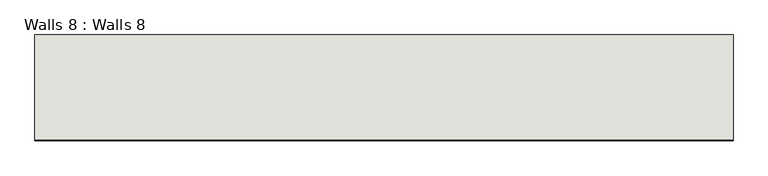
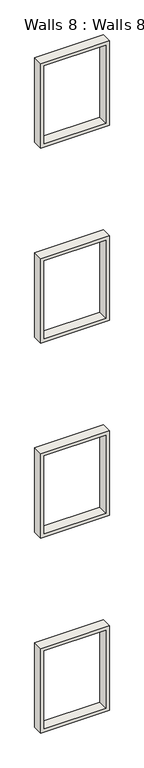
"""IFC4 building model written with IfcOpenShell, lengths in millimetres: wall geometry, Walls 8 : Walls 8."""

from ifc_helpers import new_model, si_unit, frame, origin, place, context, project, spatial, polyline, outline, extrude, source, transform, mapped, element, save


def walls_8_walls_8_31a24d2c(model_context):
    return source(origin(), model_context, "Body", "SweptSolid", [
        extrude(outline(polyline([(13030.2, 769.9073388), (13030.2, 1785.9073388), (14351.0, 1785.9073388), (14351.0, 769.9073388), (13030.2, 769.9073388)]), holes=[polyline([(13081.0, 820.7073388), (14300.2, 820.7073388), (14300.2, 1735.1073388), (13081.0, 1735.1073388), (13081.0, 820.7073388)])]), frame((0.0, -41.1211995, 0.0), z_axis=(0.0, 1.0, 0.0), x_axis=(0.0, 0.0, 1.0)), (0.0, 0.0, 1.0), 152.4),
        extrude(outline(polyline([(9982.2, 769.9073388), (9982.2, 1785.9073388), (11303.0, 1785.9073388), (11303.0, 769.9073388), (9982.2, 769.9073388)]), holes=[polyline([(10033.0, 820.7073388), (11252.2, 820.7073388), (11252.2, 1735.1073388), (10033.0, 1735.1073388), (10033.0, 820.7073388)])]), frame((0.0, -41.1211995, 0.0), z_axis=(0.0, 1.0, 0.0), x_axis=(0.0, 0.0, 1.0)), (0.0, 0.0, 1.0), 152.4),
        extrude(outline(polyline([(6934.2, 769.9073388), (6934.2, 1785.9073388), (8255.0, 1785.9073388), (8255.0, 769.9073388), (6934.2, 769.9073388)]), holes=[polyline([(6985.0, 820.7073388), (8204.2, 820.7073388), (8204.2, 1735.1073388), (6985.0, 1735.1073388), (6985.0, 820.7073388)])]), frame((0.0, -41.1211995, 0.0), z_axis=(0.0, 1.0, 0.0), x_axis=(0.0, 0.0, 1.0)), (0.0, 0.0, 1.0), 152.4),
        extrude(outline(polyline([(3886.2, 769.9073388), (3886.2, 1785.9073388), (5207.0, 1785.9073388), (5207.0, 769.9073388), (3886.2, 769.9073388)]), holes=[polyline([(3937.0, 820.7073388), (5156.2, 820.7073388), (5156.2, 1735.1073388), (3937.0, 1735.1073388), (3937.0, 820.7073388)])]), frame((0.0, -41.1211995, 0.0), z_axis=(0.0, 1.0, 0.0), x_axis=(0.0, 0.0, 1.0)), (0.0, 0.0, 1.0), 152.4),
    ])


if __name__ == "__main__":
    model = new_model("IFC4")
    model_context = context("Model", 3, world=origin())
    ifc_project = project(units=[si_unit("LENGTHUNIT", "METRE", prefix="MILLI")], contexts=[model_context])
    site = spatial("IfcSite", under=ifc_project)
    building = spatial("IfcBuilding", under=site)
    placement = place(None, origin())
    walls_8_walls_8_shape = walls_8_walls_8_31a24d2c(model_context)
    element("IfcWall", 1, ObjectType="Walls 8 : Walls 8", at=placement, inside=building, context=model_context, shape_type="MappedRepresentation", body=[
        mapped(walls_8_walls_8_shape, transform((0.0, 0.0, 0.0), x_axis=(1.0, 0.0, 0.0), y_axis=(0.0, 1.0, 0.0), z_axis=(0.0, 0.0, 1.0))),
    ])
    save(model, "model.ifc")

# Revit data of these elements
# Element 1 (IfcWall, "Walls 8 : Walls 8")
#   Materials on its faces: "1 wall white", "Default Wall"
# Materials
#   "1 wall white": class "Generic", colour RGB 244 245 241, transparency 0, Cost = 0
#   "Default Wall": colour RGB 128 128 128, transparency 0, Cost = 0
